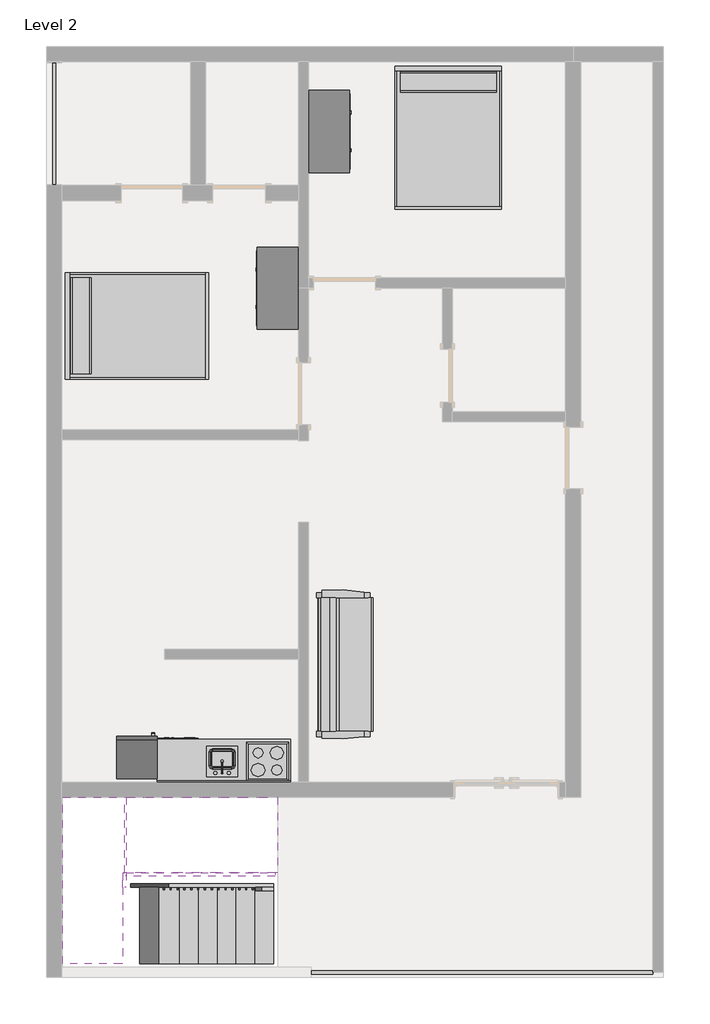
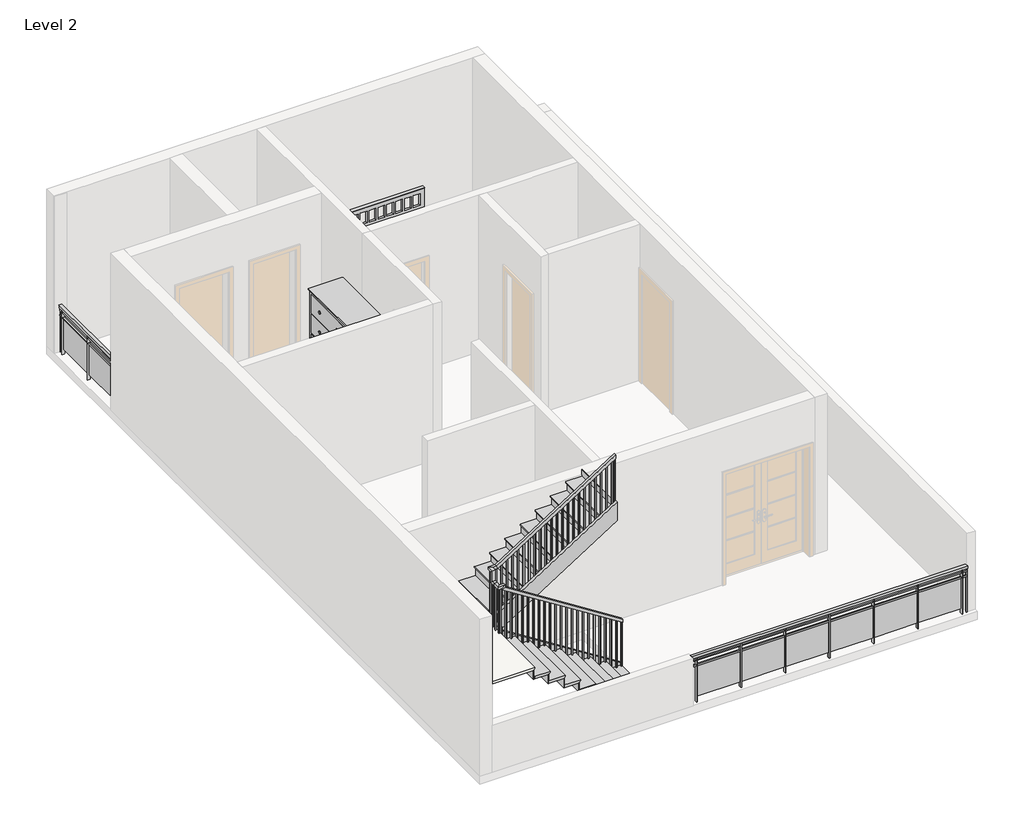
# One storey, part 2 of 2: 6 furniture elements, 4 proxies, 3 members, 3 railings, 2 stair flights, 1 flow terminal, 1 slab.
"""IFC4 building model written with IfcOpenShell, lengths in millimetres."""

from ifc_helpers import new_model, si_unit, frame, origin, place, context, project, spatial, polyline, outline, extrude, faceted_brep, transform, mapped, element, save
from components import proxy_a6faaae8, proxy_45b28599, kitchenette_medium_kitchenette_medium_844211aa, proxy_c523a7b7, flow_terminal_871c2e40, furniture_35c09872, furniture_c6510c7c, furniture_9fa109b2, furniture_aff9b2fb, non_monolithic_landing_077bd761, stair_flight_3c50d200, stair_flight_53bbb6a0

model = new_model("IFC4")

# Units and contexts
model_context = context("Model", 3, world=origin())
ifc_project = project(units=[si_unit("LENGTHUNIT", "METRE", prefix="MILLI")], contexts=[model_context])

# Site, building, storey
site = spatial("IfcSite", under=ifc_project)
building = spatial("IfcBuilding", under=site)
storey = spatial("IfcBuildingStorey", under=building, Name="Level 2", Elevation=3200.4)

# Proxies
placement = place(None, origin())
proxy_shape = proxy_a6faaae8(model_context)
element("IfcBuildingElementProxy", 1, Name="Cook Top-4 Unit2 : 22\" x 20\"", ObjectType="Cook Top-4 Unit2 : 22\" x 20\"", at=placement, inside=storey, context=model_context, shape_type="MappedRepresentation", body=[
    mapped(proxy_shape, transform((-8075.1683044, -841.1891189, 3200.4), x_axis=(-1.0000000000000004, 0.0, 0.0), y_axis=(0.0, -1.0000000000000004, 0.0), z_axis=(0.0, 0.0, 1.0))),
])
proxy_2_shape = proxy_45b28599(model_context)
element("IfcBuildingElementProxy", 2, Name="Dishwasher : 24\" x 24\" x 34\"", ObjectType="Dishwasher : 24\" x 24\" x 34\"", at=placement, inside=storey, context=model_context, shape_type="MappedRepresentation", body=[
    mapped(proxy_2_shape, transform((-9026.3508359, -549.3395541, 3200.4), x_axis=(-1.0000000000000004, 0.0, 0.0), y_axis=(0.0, -1.0000000000000004, 0.0), z_axis=(0.0, 0.0, 1.0))),
])
kitchenette_medium_kitchenette_medium_shape = kitchenette_medium_kitchenette_medium_844211aa(model_context)
element("IfcBuildingElementProxy", 3, Name="Kitchenette - Medium : Kitchenette - Medium", ObjectType="Kitchenette - Medium : Kitchenette - Medium", at=placement, inside=storey, context=model_context, shape_type="MappedRepresentation", body=[
    mapped(kitchenette_medium_kitchenette_medium_shape, transform((-8399.3305994, -1145.9891189, 3200.4), x_axis=(-1.0000000000000004, 0.0, 0.0), y_axis=(0.0, -1.0000000000000004, 0.0), z_axis=(0.0, 0.0, 1.0))),
])
proxy_3_shape = proxy_c523a7b7(model_context)
element("IfcBuildingElementProxy", 4, Name="Refrigerator : 24\" x 25\" LH", ObjectType="Refrigerator : 24\" x 25\" LH", at=placement, inside=storey, context=model_context, shape_type="MappedRepresentation", body=[
    mapped(proxy_3_shape, transform((-10011.9183044, -795.5401474, 3200.4), x_axis=(-1.0000000000000004, 0.0, 0.0), y_axis=(0.0, -1.0000000000000004, 0.0), z_axis=(0.0, 0.0, 1.0))),
])

# Flow terminal
flow_terminal_shape = flow_terminal_871c2e40(model_context)
element("IfcFlowTerminal", 5, ObjectType="Sink Kitchen-Island : 18\" x 18\"", at=placement, inside=storey, context=model_context, shape_type="MappedRepresentation", body=[
    mapped(flow_terminal_shape, transform((-8732.5790638, -838.8437178, 3186.0), x_axis=(-1.0000000000000004, 0.0, 0.0), y_axis=(0.0, -1.0000000000000004, 0.0), z_axis=(0.0, 0.0, 1.0))),
])

# Furniture
furniture_shape = furniture_35c09872(model_context)
element("IfcFurniture", 6, ObjectType="Bed-Shaker : Queen 62\" x 83\"", at=placement, inside=storey, context=model_context, shape_type="MappedRepresentation", body=[
    mapped(furniture_shape, transform((-11059.6683044, 5629.4608811, 3200.4), x_axis=(0.0, 1.0, 0.0), y_axis=(-1.0, 0.0, 0.0), z_axis=(0.0, 0.0, 1.0))),
])
element("IfcFurniture", 7, ObjectType="Bed-Shaker : Queen 62\" x 83\"", at=placement, inside=storey, context=model_context, shape_type="MappedRepresentation", body=[
    mapped(furniture_shape, transform((-5376.4183044, 9445.8108811, 3200.4), x_axis=(1.0, 0.0, 0.0), y_axis=(0.0, 1.0, 0.0), z_axis=(0.0, 0.0, 1.0))),
])
furniture_2_shape = furniture_c6510c7c(model_context)
element("IfcFurniture", 8, ObjectType="Counter Top w Sink Hole : 24\" Depth", at=placement, inside=storey, context=model_context, shape_type="MappedRepresentation", body=[
    mapped(furniture_2_shape, transform((-8932.7305994, -1145.9891189, 3186.0), x_axis=(-1.0000000000000004, 0.0, 0.0), y_axis=(0.0, -1.0000000000000004, 0.0), z_axis=(0.0, 0.0, 1.0))),
])
furniture_3_shape = furniture_9fa109b2(model_context)
element("IfcFurniture", 9, ObjectType="Dresser : 48\" x 72\" x 24\"", at=placement, inside=storey, context=model_context, shape_type="MappedRepresentation", body=[
    mapped(furniture_3_shape, transform((-7559.6053503, 5900.0176213, 3200.4), x_axis=(0.0, -1.0000000000000004, 0.0), y_axis=(1.0000000000000004, 0.0, 0.0), z_axis=(0.0, 0.0, 1.0))),
])
element("IfcFurniture", 10, ObjectType="Dresser : 48\" x 72\" x 24\"", at=placement, inside=storey, context=model_context, shape_type="MappedRepresentation", body=[
    mapped(furniture_3_shape, transform((-7523.9312585, 8762.5041409, 3200.4), x_axis=(0.0, 1.0000000000000009, 0.0), y_axis=(-1.0000000000000009, 0.0, 0.0), z_axis=(0.0, 0.0, 1.0))),
])
furniture_4_shape = furniture_aff9b2fb(model_context)
element("IfcFurniture", 11, ObjectType="Sofa-Pensi : 84\"", at=placement, inside=storey, context=model_context, shape_type="MappedRepresentation", body=[
    mapped(furniture_4_shape, transform((-6655.0584683, 315.3046311, 3200.4), x_axis=(0.0, 1.0, 0.0), y_axis=(-1.0, 0.0, 0.0), z_axis=(0.0, 0.0, 1.0))),
])

# Members
element("IfcMember", 12, ObjectType="Stringer - 2\" Width", at=placement, inside=storey, context=model_context, shape_type="SweptSolid", body=[
    extrude(outline(polyline([(3200.4, -7986.2683044), (3415.4106437, -7986.2683044), (4805.483371, -10170.6683044), (4444.2010268, -10170.6683044), (3200.4, -8216.1238337), (3200.4, -7986.2683044)])), frame((0.0, -2706.1923176, 0.0), z_axis=(0.0, 1.0, 0.0), x_axis=(0.0, 0.0, 1.0)), (0.0, 0.0, 1.0), 50.8),
])
element("IfcMember", 13, ObjectType="Stringer - 2\" Width", at=placement, inside=storey, context=model_context, shape_type="SweptSolid", body=[
    extrude(outline(polyline([(5031.7742801, -10170.6683044), (4670.4919359, -10170.6683044), (6076.7282995, -7960.8683044), (6438.0106437, -7960.8683044), (5031.7742801, -10170.6683044)])), frame((0.0, -2542.9891189, 0.0), z_axis=(0.0, 1.0, 0.0), x_axis=(0.0, 0.0, 1.0)), (0.0, 0.0, 1.0), 50.8),
])
element("IfcMember", 14, ObjectType="Stringer - 2\" Width", at=placement, inside=storey, context=model_context, shape_type="SweptSolid", body=[
    extrude(outline(polyline([(-10170.6683044, -2706.1923176), (-10221.4683044, -2706.1923176), (-10221.4683044, -2492.1891189), (-10170.6683044, -2492.1891189), (-10170.6683044, -2706.1923176)])), frame((0.0, 0.0, 4572.0), z_axis=(0.0, 0.0, 1.0), x_axis=(1.0, 0.0, 0.0)), (0.0, 0.0, 1.0), 304.8),
])

# Railings
element("IfcRailing", 15, ObjectType="Glass Panel - Bottom Fill", at=placement, inside=storey, context=model_context, shape_type="SweptSolid", body=[
    extrude(outline(polyline([(-7427.4683044, -3990.7891189), (-7427.4683044, -3939.9891189), (-2360.1683044, -3939.9891189), (-2360.1683044, -3990.7891189), (-7427.4683044, -3990.7891189)])), frame((0.0, 0.0, 4064.0), z_axis=(0.0, 0.0, 1.0), x_axis=(1.0, 0.0, 0.0)), (0.0, 0.0, 1.0), 50.8),
    extrude(outline(polyline([(-7427.4683044, -3978.0891189), (-7427.4683044, -3952.6891189), (-2360.1683044, -3952.6891189), (-2360.1683044, -3978.0891189), (-7427.4683044, -3978.0891189)])), frame((0.0, 0.0, 4000.5), z_axis=(0.0, 0.0, 1.0), x_axis=(1.0, 0.0, 0.0)), (0.0, 0.0, 1.0), 25.4),
    extrude(outline(polyline([(-7427.4683044, -3978.0891189), (-7427.4683044, -3952.6891189), (-2360.1683044, -3952.6891189), (-2360.1683044, -3978.0891189), (-7427.4683044, -3978.0891189)])), frame((0.0, 0.0, 3898.9), z_axis=(0.0, 0.0, 1.0), x_axis=(1.0, 0.0, 0.0)), (0.0, 0.0, 1.0), 25.4),
    extrude(outline(polyline([(-2461.7683044, -3990.7891189), (-2461.7683044, -3939.9891189), (-2449.0683044, -3939.9891189), (-2449.0683044, -3990.7891189), (-2461.7683044, -3990.7891189)])), frame((0.0, 0.0, 3200.4), z_axis=(0.0, 0.0, 1.0), x_axis=(1.0, 0.0, 0.0)), (0.0, 0.0, 1.0), 863.6),
    extrude(outline(polyline([(-3268.2183044, -3958.8539619), (-2455.4183044, -3958.8539619), (-2455.4183044, -3965.2039619), (-3268.2183044, -3965.2039619), (-3268.2183044, -3958.8539619)])), frame((0.0, 0.0, 3302.0), z_axis=(0.0, 0.0, 1.0), x_axis=(1.0, 0.0, 0.0)), (0.0, 0.0, 1.0), 596.9),
    extrude(outline(polyline([(-3274.5683044, -3990.7891189), (-3274.5683044, -3939.9891189), (-3261.8683044, -3939.9891189), (-3261.8683044, -3990.7891189), (-3274.5683044, -3990.7891189)])), frame((0.0, 0.0, 3200.4), z_axis=(0.0, 0.0, 1.0), x_axis=(1.0, 0.0, 0.0)), (0.0, 0.0, 1.0), 863.6),
    extrude(outline(polyline([(-4081.0183044, -3958.8539619), (-3268.2183044, -3958.8539619), (-3268.2183044, -3965.2039619), (-4081.0183044, -3965.2039619), (-4081.0183044, -3958.8539619)])), frame((0.0, 0.0, 3302.0), z_axis=(0.0, 0.0, 1.0), x_axis=(1.0, 0.0, 0.0)), (0.0, 0.0, 1.0), 596.9),
    extrude(outline(polyline([(-4087.3683044, -3990.7891189), (-4087.3683044, -3939.9891189), (-4074.6683044, -3939.9891189), (-4074.6683044, -3990.7891189), (-4087.3683044, -3990.7891189)])), frame((0.0, 0.0, 3200.4), z_axis=(0.0, 0.0, 1.0), x_axis=(1.0, 0.0, 0.0)), (0.0, 0.0, 1.0), 863.6),
    extrude(outline(polyline([(-4893.8183044, -3958.8539619), (-4081.0183044, -3958.8539619), (-4081.0183044, -3965.2039619), (-4893.8183044, -3965.2039619), (-4893.8183044, -3958.8539619)])), frame((0.0, 0.0, 3302.0), z_axis=(0.0, 0.0, 1.0), x_axis=(1.0, 0.0, 0.0)), (0.0, 0.0, 1.0), 596.9),
    extrude(outline(polyline([(-4900.1683044, -3990.7891189), (-4900.1683044, -3939.9891189), (-4887.4683044, -3939.9891189), (-4887.4683044, -3990.7891189), (-4900.1683044, -3990.7891189)])), frame((0.0, 0.0, 3200.4), z_axis=(0.0, 0.0, 1.0), x_axis=(1.0, 0.0, 0.0)), (0.0, 0.0, 1.0), 863.6),
    extrude(outline(polyline([(-5706.6183044, -3958.8539619), (-4893.8183044, -3958.8539619), (-4893.8183044, -3965.2039619), (-5706.6183044, -3965.2039619), (-5706.6183044, -3958.8539619)])), frame((0.0, 0.0, 3302.0), z_axis=(0.0, 0.0, 1.0), x_axis=(1.0, 0.0, 0.0)), (0.0, 0.0, 1.0), 596.9),
    extrude(outline(polyline([(-5712.9683044, -3990.7891189), (-5712.9683044, -3939.9891189), (-5700.2683044, -3939.9891189), (-5700.2683044, -3990.7891189), (-5712.9683044, -3990.7891189)])), frame((0.0, 0.0, 3200.4), z_axis=(0.0, 0.0, 1.0), x_axis=(1.0, 0.0, 0.0)), (0.0, 0.0, 1.0), 863.6),
    extrude(outline(polyline([(-6519.4183044, -3958.8539619), (-5706.6183044, -3958.8539619), (-5706.6183044, -3965.2039619), (-6519.4183044, -3965.2039619), (-6519.4183044, -3958.8539619)])), frame((0.0, 0.0, 3302.0), z_axis=(0.0, 0.0, 1.0), x_axis=(1.0, 0.0, 0.0)), (0.0, 0.0, 1.0), 596.9),
    extrude(outline(polyline([(-6525.7683044, -3990.7891189), (-6525.7683044, -3939.9891189), (-6513.0683044, -3939.9891189), (-6513.0683044, -3990.7891189), (-6525.7683044, -3990.7891189)])), frame((0.0, 0.0, 3200.4), z_axis=(0.0, 0.0, 1.0), x_axis=(1.0, 0.0, 0.0)), (0.0, 0.0, 1.0), 863.6),
    extrude(outline(polyline([(-7332.2183044, -3958.8539619), (-6519.4183044, -3958.8539619), (-6519.4183044, -3965.2039619), (-7332.2183044, -3965.2039619), (-7332.2183044, -3958.8539619)])), frame((0.0, 0.0, 3302.0), z_axis=(0.0, 0.0, 1.0), x_axis=(1.0, 0.0, 0.0)), (0.0, 0.0, 1.0), 596.9),
    extrude(outline(polyline([(-7338.5683044, -3990.7891189), (-7338.5683044, -3939.9891189), (-7325.8683044, -3939.9891189), (-7325.8683044, -3990.7891189), (-7338.5683044, -3990.7891189)])), frame((0.0, 0.0, 3200.4), z_axis=(0.0, 0.0, 1.0), x_axis=(1.0, 0.0, 0.0)), (0.0, 0.0, 1.0), 863.6),
    extrude(outline(polyline([(-2372.8683044, -3974.9141189), (-2372.8683044, -3955.8641189), (-2353.8183044, -3955.8641189), (-2353.8183044, -3974.9141189), (-2372.8683044, -3974.9141189)])), frame((0.0, 0.0, 3200.4), z_axis=(0.0, 0.0, 1.0), x_axis=(1.0, 0.0, 0.0)), (0.0, 0.0, 1.0), 863.6),
    extrude(outline(polyline([(-7433.8183044, -3974.9141189), (-7433.8183044, -3955.8641189), (-7414.7683044, -3955.8641189), (-7414.7683044, -3974.9141189), (-7433.8183044, -3974.9141189)])), frame((0.0, 0.0, 3200.4), z_axis=(0.0, 0.0, 1.0), x_axis=(1.0, 0.0, 0.0)), (0.0, 0.0, 1.0), 863.6),
])
element("IfcRailing", 16, ObjectType="Glass Panel - Bottom Fill", at=placement, inside=storey, context=model_context, shape_type="SweptSolid", body=[
    extrude(outline(polyline([(-11262.8683044, 9509.3108811), (-11212.0683044, 9509.3108811), (-11212.0683044, 7705.9108811), (-11262.8683044, 7705.9108811), (-11262.8683044, 9509.3108811)])), frame((0.0, 0.0, 4064.0), z_axis=(0.0, 0.0, 1.0), x_axis=(1.0, 0.0, 0.0)), (0.0, 0.0, 1.0), 50.8),
    extrude(outline(polyline([(-11250.1683044, 9509.3108811), (-11224.7683044, 9509.3108811), (-11224.7683044, 7705.9108811), (-11250.1683044, 7705.9108811), (-11250.1683044, 9509.3108811)])), frame((0.0, 0.0, 4000.5), z_axis=(0.0, 0.0, 1.0), x_axis=(1.0, 0.0, 0.0)), (0.0, 0.0, 1.0), 25.4),
    extrude(outline(polyline([(-11250.1683044, 9509.3108811), (-11224.7683044, 9509.3108811), (-11224.7683044, 7705.9108811), (-11250.1683044, 7705.9108811), (-11250.1683044, 9509.3108811)])), frame((0.0, 0.0, 3898.9), z_axis=(0.0, 0.0, 1.0), x_axis=(1.0, 0.0, 0.0)), (0.0, 0.0, 1.0), 25.4),
    extrude(outline(polyline([(-11262.8683044, 7801.1608811), (-11212.0683044, 7801.1608811), (-11212.0683044, 7788.4608811), (-11262.8683044, 7788.4608811), (-11262.8683044, 7801.1608811)])), frame((0.0, 0.0, 3200.4), z_axis=(0.0, 0.0, 1.0), x_axis=(1.0, 0.0, 0.0)), (0.0, 0.0, 1.0), 863.6),
    extrude(outline(polyline([(-11230.9331474, 8607.6108811), (-11230.9331474, 7794.8108811), (-11237.2831474, 7794.8108811), (-11237.2831474, 8607.6108811), (-11230.9331474, 8607.6108811)])), frame((0.0, 0.0, 3302.0), z_axis=(0.0, 0.0, 1.0), x_axis=(1.0, 0.0, 0.0)), (0.0, 0.0, 1.0), 596.9),
    extrude(outline(polyline([(-11262.8683044, 8613.9608811), (-11212.0683044, 8613.9608811), (-11212.0683044, 8601.2608811), (-11262.8683044, 8601.2608811), (-11262.8683044, 8613.9608811)])), frame((0.0, 0.0, 3200.4), z_axis=(0.0, 0.0, 1.0), x_axis=(1.0, 0.0, 0.0)), (0.0, 0.0, 1.0), 863.6),
    extrude(outline(polyline([(-11230.9331474, 9420.4108811), (-11230.9331474, 8607.6108811), (-11237.2831474, 8607.6108811), (-11237.2831474, 9420.4108811), (-11230.9331474, 9420.4108811)])), frame((0.0, 0.0, 3302.0), z_axis=(0.0, 0.0, 1.0), x_axis=(1.0, 0.0, 0.0)), (0.0, 0.0, 1.0), 596.9),
    extrude(outline(polyline([(-11262.8683044, 9426.7608811), (-11212.0683044, 9426.7608811), (-11212.0683044, 9414.0608811), (-11262.8683044, 9414.0608811), (-11262.8683044, 9426.7608811)])), frame((0.0, 0.0, 3200.4), z_axis=(0.0, 0.0, 1.0), x_axis=(1.0, 0.0, 0.0)), (0.0, 0.0, 1.0), 863.6),
    extrude(outline(polyline([(-11246.9933044, 7718.6108811), (-11227.9433044, 7718.6108811), (-11227.9433044, 7699.5608811), (-11246.9933044, 7699.5608811), (-11246.9933044, 7718.6108811)])), frame((0.0, 0.0, 3200.4), z_axis=(0.0, 0.0, 1.0), x_axis=(1.0, 0.0, 0.0)), (0.0, 0.0, 1.0), 863.6),
    extrude(outline(polyline([(-11246.9933044, 9515.6608811), (-11227.9433044, 9515.6608811), (-11227.9433044, 9496.6108811), (-11246.9933044, 9496.6108811), (-11246.9933044, 9515.6608811)])), frame((0.0, 0.0, 3200.4), z_axis=(0.0, 0.0, 1.0), x_axis=(1.0, 0.0, 0.0)), (0.0, 0.0, 1.0), 863.6),
])
element("IfcRailing", 17, ObjectType="Handrail - Rectangular", at=placement, inside=storey, context=model_context, shape_type="SolidModel", body=[
    faceted_brep([(-7986.2683044, -2756.9923176, 4292.6), (-7986.2683044, -2756.9923176, 4232.386276), (-7986.2683044, -2706.1923176, 4232.386276), (-7986.2683044, -2706.1923176, 4292.6), (-10145.2683044, -2756.9923176, 5666.5090909), (-10196.0683044, -2756.9923176, 5638.6226396), (-10196.0683044, -2706.1923176, 5638.6226396), (-10145.2683044, -2706.1923176, 5666.5090909), (-10145.2683044, -2756.9923176, 5715.0), (-10196.0683044, -2756.9923176, 5664.2), (-10196.0683044, -2706.1923176, 5664.2), (-10145.2683044, -2706.1923176, 5715.0), (-10272.2683044, -2756.9923176, 5715.0), (-10272.2683044, -2756.9923176, 5664.2), (-10221.4683044, -2706.1923176, 5664.2), (-10221.4683044, -2706.1923176, 5715.0), (-10272.2683044, -2629.9923176, 5715.0), (-10272.2683044, -2629.9923176, 5664.2), (-10221.4683044, -2629.9923176, 5664.2), (-10221.4683044, -2629.9923176, 5715.0), (-10272.2683044, -2568.3891189, 5715.0), (-10272.2683044, -2517.5891189, 5664.2), (-10221.4683044, -2517.5891189, 5664.2), (-10221.4683044, -2568.3891189, 5715.0), (-10272.2683044, -2568.3891189, 5925.1272727), (-10272.2683044, -2517.5891189, 5874.3272727), (-10221.4683044, -2517.5891189, 5874.3272727), (-10221.4683044, -2568.3891189, 5925.1272727), (-7960.8683044, -2441.3891189, 7315.2), (-7960.8683044, -2492.1891189, 7315.2), (-7960.8683044, -2492.1891189, 7254.986276), (-7960.8683044, -2441.3891189, 7254.986276), (-10130.4753095, -2441.3891189, 5874.3272727), (-10145.2683044, -2441.3891189, 5925.1272727), (-10130.4753095, -2492.1891189, 5874.3272727), (-10145.2683044, -2492.1891189, 5925.1272727), (-10272.2683044, -2441.3891189, 5925.1272727), (-10272.2683044, -2441.3891189, 5874.3272727), (-10221.4683044, -2492.1891189, 5874.3272727), (-10221.4683044, -2492.1891189, 5925.1272727)], [[[0, 1, 2, 3]], [[1, 0, 4, 5]], [[2, 1, 5, 6]], [[3, 2, 6, 7]], [[0, 3, 7, 4]], [[5, 4, 8, 9]], [[6, 5, 9, 10]], [[7, 6, 10, 11]], [[4, 7, 11, 8]], [[9, 8, 12, 13]], [[10, 9, 13, 14]], [[11, 10, 14, 15]], [[8, 11, 15, 12]], [[13, 12, 16, 17]], [[14, 13, 17, 18]], [[15, 14, 18, 19]], [[12, 15, 19, 16]], [[17, 16, 20, 21]], [[18, 17, 21, 22]], [[19, 18, 22, 23]], [[16, 19, 23, 20]], [[21, 20, 24, 25]], [[22, 21, 25, 26]], [[23, 22, 26, 27]], [[20, 23, 27, 24]], [[28, 29, 30, 31]], [[32, 33, 28, 31]], [[34, 32, 31, 30]], [[35, 34, 30, 29]], [[33, 35, 29, 28]], [[25, 24, 36, 37]], [[26, 25, 37, 38]], [[27, 26, 38, 39]], [[24, 27, 39, 36]], [[37, 36, 33, 32]], [[38, 37, 32, 34]], [[39, 38, 34, 35]], [[36, 39, 35, 33]]]),
    extrude(outline(polyline([(7228.7203669, -8002.1433044), (7216.5976396, -8021.1933044), (6223.0, -8021.1933044), (6223.0, -8002.1433044), (7228.7203669, -8002.1433044)])), frame((0.0, -2476.3141189, 0.0), z_axis=(0.0, 1.0, 0.0), x_axis=(0.0, 0.0, 1.0)), (0.0, 0.0, 1.0), 19.05),
    extrude(outline(polyline([(7164.0658214, -8103.7433044), (7151.9430941, -8122.7933044), (6223.0, -8122.7933044), (6223.0, -8103.7433044), (7164.0658214, -8103.7433044)])), frame((0.0, -2476.3141189, 0.0), z_axis=(0.0, 1.0, 0.0), x_axis=(0.0, 0.0, 1.0)), (0.0, 0.0, 1.0), 19.05),
    extrude(outline(polyline([(7099.411276, -8205.3433044), (7087.2885487, -8224.3933044), (6223.0, -8224.3933044), (6223.0, -8205.3433044), (7099.411276, -8205.3433044)])), frame((0.0, -2476.3141189, 0.0), z_axis=(0.0, 1.0, 0.0), x_axis=(0.0, 0.0, 1.0)), (0.0, 0.0, 1.0), 19.05),
    extrude(outline(polyline([(7034.7567305, -8306.9433044), (7022.6340032, -8325.9933044), (6045.2, -8325.9933044), (6045.2, -8306.9433044), (7034.7567305, -8306.9433044)])), frame((0.0, -2476.3141189, 0.0), z_axis=(0.0, 1.0, 0.0), x_axis=(0.0, 0.0, 1.0)), (0.0, 0.0, 1.0), 19.05),
    extrude(outline(polyline([(6970.1021851, -8408.5433044), (6957.9794578, -8427.5933044), (6045.2, -8427.5933044), (6045.2, -8408.5433044), (6970.1021851, -8408.5433044)])), frame((0.0, -2476.3141189, 0.0), z_axis=(0.0, 1.0, 0.0), x_axis=(0.0, 0.0, 1.0)), (0.0, 0.0, 1.0), 19.05),
    extrude(outline(polyline([(6905.4476396, -8510.1433044), (6893.3249123, -8529.1933044), (6045.2, -8529.1933044), (6045.2, -8510.1433044), (6905.4476396, -8510.1433044)])), frame((0.0, -2476.3141189, 0.0), z_axis=(0.0, 1.0, 0.0), x_axis=(0.0, 0.0, 1.0)), (0.0, 0.0, 1.0), 19.05),
    extrude(outline(polyline([(6840.7930941, -8611.7433044), (6828.6703669, -8630.7933044), (5867.4, -8630.7933044), (5867.4, -8611.7433044), (6840.7930941, -8611.7433044)])), frame((0.0, -2476.3141189, 0.0), z_axis=(0.0, 1.0, 0.0), x_axis=(0.0, 0.0, 1.0)), (0.0, 0.0, 1.0), 19.05),
    extrude(outline(polyline([(6776.1385487, -8713.3433044), (6764.0158214, -8732.3933044), (5867.4, -8732.3933044), (5867.4, -8713.3433044), (6776.1385487, -8713.3433044)])), frame((0.0, -2476.3141189, 0.0), z_axis=(0.0, 1.0, 0.0), x_axis=(0.0, 0.0, 1.0)), (0.0, 0.0, 1.0), 19.05),
    extrude(outline(polyline([(6711.4840032, -8814.9433044), (6699.361276, -8833.9933044), (5689.6, -8833.9933044), (5689.6, -8814.9433044), (6711.4840032, -8814.9433044)])), frame((0.0, -2476.3141189, 0.0), z_axis=(0.0, 1.0, 0.0), x_axis=(0.0, 0.0, 1.0)), (0.0, 0.0, 1.0), 19.05),
    extrude(outline(polyline([(6646.8294578, -8916.5433044), (6634.7067305, -8935.5933044), (5689.6, -8935.5933044), (5689.6, -8916.5433044), (6646.8294578, -8916.5433044)])), frame((0.0, -2476.3141189, 0.0), z_axis=(0.0, 1.0, 0.0), x_axis=(0.0, 0.0, 1.0)), (0.0, 0.0, 1.0), 19.05),
    extrude(outline(polyline([(6582.1749123, -9018.1433044), (6570.0521851, -9037.1933044), (5689.6, -9037.1933044), (5689.6, -9018.1433044), (6582.1749123, -9018.1433044)])), frame((0.0, -2476.3141189, 0.0), z_axis=(0.0, 1.0, 0.0), x_axis=(0.0, 0.0, 1.0)), (0.0, 0.0, 1.0), 19.05),
    extrude(outline(polyline([(6517.5203669, -9119.7433044), (6505.3976396, -9138.7933044), (5511.8, -9138.7933044), (5511.8, -9119.7433044), (6517.5203669, -9119.7433044)])), frame((0.0, -2476.3141189, 0.0), z_axis=(0.0, 1.0, 0.0), x_axis=(0.0, 0.0, 1.0)), (0.0, 0.0, 1.0), 19.05),
    extrude(outline(polyline([(6452.8658214, -9221.3433044), (6440.7430941, -9240.3933044), (5511.8, -9240.3933044), (5511.8, -9221.3433044), (6452.8658214, -9221.3433044)])), frame((0.0, -2476.3141189, 0.0), z_axis=(0.0, 1.0, 0.0), x_axis=(0.0, 0.0, 1.0)), (0.0, 0.0, 1.0), 19.05),
    extrude(outline(polyline([(6388.211276, -9322.9433044), (6376.0885487, -9341.9933044), (5511.8, -9341.9933044), (5511.8, -9322.9433044), (6388.211276, -9322.9433044)])), frame((0.0, -2476.3141189, 0.0), z_axis=(0.0, 1.0, 0.0), x_axis=(0.0, 0.0, 1.0)), (0.0, 0.0, 1.0), 19.05),
    extrude(outline(polyline([(6323.5567305, -9424.5433044), (6311.4340032, -9443.5933044), (5334.0, -9443.5933044), (5334.0, -9424.5433044), (6323.5567305, -9424.5433044)])), frame((0.0, -2476.3141189, 0.0), z_axis=(0.0, 1.0, 0.0), x_axis=(0.0, 0.0, 1.0)), (0.0, 0.0, 1.0), 19.05),
    extrude(outline(polyline([(6258.9021851, -9526.1433044), (6246.7794578, -9545.1933044), (5334.0, -9545.1933044), (5334.0, -9526.1433044), (6258.9021851, -9526.1433044)])), frame((0.0, -2476.3141189, 0.0), z_axis=(0.0, 1.0, 0.0), x_axis=(0.0, 0.0, 1.0)), (0.0, 0.0, 1.0), 19.05),
    extrude(outline(polyline([(6194.2476396, -9627.7433044), (6182.1249123, -9646.7933044), (5334.0, -9646.7933044), (5334.0, -9627.7433044), (6194.2476396, -9627.7433044)])), frame((0.0, -2476.3141189, 0.0), z_axis=(0.0, 1.0, 0.0), x_axis=(0.0, 0.0, 1.0)), (0.0, 0.0, 1.0), 19.05),
    extrude(outline(polyline([(6129.5930941, -9729.3433044), (6117.4703669, -9748.3933044), (5156.2, -9748.3933044), (5156.2, -9729.3433044), (6129.5930941, -9729.3433044)])), frame((0.0, -2476.3141189, 0.0), z_axis=(0.0, 1.0, 0.0), x_axis=(0.0, 0.0, 1.0)), (0.0, 0.0, 1.0), 19.05),
    extrude(outline(polyline([(6064.9385487, -9830.9433044), (6052.8158214, -9849.9933044), (5156.2, -9849.9933044), (5156.2, -9830.9433044), (6064.9385487, -9830.9433044)])), frame((0.0, -2476.3141189, 0.0), z_axis=(0.0, 1.0, 0.0), x_axis=(0.0, 0.0, 1.0)), (0.0, 0.0, 1.0), 19.05),
    extrude(outline(polyline([(6000.2840032, -9932.5433044), (5988.161276, -9951.5933044), (4978.4, -9951.5933044), (4978.4, -9932.5433044), (6000.2840032, -9932.5433044)])), frame((0.0, -2476.3141189, 0.0), z_axis=(0.0, 1.0, 0.0), x_axis=(0.0, 0.0, 1.0)), (0.0, 0.0, 1.0), 19.05),
    extrude(outline(polyline([(5935.6294578, -10034.1433044), (5923.5067305, -10053.1933044), (4978.4, -10053.1933044), (4978.4, -10034.1433044), (5935.6294578, -10034.1433044)])), frame((0.0, -2476.3141189, 0.0), z_axis=(0.0, 1.0, 0.0), x_axis=(0.0, 0.0, 1.0)), (0.0, 0.0, 1.0), 19.05),
    extrude(outline(polyline([(-10154.7933044, -2476.3141189), (-10154.7933044, -2457.2641189), (-10135.7433044, -2457.2641189), (-10135.7433044, -2476.3141189), (-10154.7933044, -2476.3141189)])), frame((0.0, 0.0, 4978.4), z_axis=(0.0, 0.0, 1.0), x_axis=(1.0, 0.0, 0.0)), (0.0, 0.0, 1.0), 895.9272727),
    extrude(outline(polyline([(-10237.3433044, -2537.9173176), (-10256.3933044, -2537.9173176), (-10256.3933044, -2518.8673176), (-10237.3433044, -2518.8673176), (-10237.3433044, -2537.9173176)])), frame((0.0, 0.0, 4800.6), z_axis=(0.0, 0.0, 1.0), x_axis=(1.0, 0.0, 0.0)), (0.0, 0.0, 1.0), 863.6),
    extrude(outline(polyline([(-10237.3433044, -2639.5173176), (-10256.3933044, -2639.5173176), (-10256.3933044, -2620.4673176), (-10237.3433044, -2620.4673176), (-10237.3433044, -2639.5173176)])), frame((0.0, 0.0, 4800.6), z_axis=(0.0, 0.0, 1.0), x_axis=(1.0, 0.0, 0.0)), (0.0, 0.0, 1.0), 863.6),
    extrude(outline(polyline([(5584.0703669, -10110.3433044), (5596.1930941, -10129.3933044), (4622.8, -10129.3933044), (4622.8, -10110.3433044), (5584.0703669, -10110.3433044)])), frame((0.0, -2741.1173176, 0.0), z_axis=(0.0, 1.0, 0.0), x_axis=(0.0, 0.0, 1.0)), (0.0, 0.0, 1.0), 19.05),
    extrude(outline(polyline([(5519.4158214, -10008.7433044), (5531.5385487, -10027.7933044), (4622.8, -10027.7933044), (4622.8, -10008.7433044), (5519.4158214, -10008.7433044)])), frame((0.0, -2741.1173176, 0.0), z_axis=(0.0, 1.0, 0.0), x_axis=(0.0, 0.0, 1.0)), (0.0, 0.0, 1.0), 19.05),
    extrude(outline(polyline([(5454.761276, -9907.1433044), (5466.8840032, -9926.1933044), (4445.0, -9926.1933044), (4445.0, -9907.1433044), (5454.761276, -9907.1433044)])), frame((0.0, -2741.1173176, 0.0), z_axis=(0.0, 1.0, 0.0), x_axis=(0.0, 0.0, 1.0)), (0.0, 0.0, 1.0), 19.05),
    extrude(outline(polyline([(5390.1067305, -9805.5433044), (5402.2294578, -9824.5933044), (4445.0, -9824.5933044), (4445.0, -9805.5433044), (5390.1067305, -9805.5433044)])), frame((0.0, -2741.1173176, 0.0), z_axis=(0.0, 1.0, 0.0), x_axis=(0.0, 0.0, 1.0)), (0.0, 0.0, 1.0), 19.05),
    extrude(outline(polyline([(5325.4521851, -9703.9433044), (5337.5749123, -9722.9933044), (4445.0, -9722.9933044), (4445.0, -9703.9433044), (5325.4521851, -9703.9433044)])), frame((0.0, -2741.1173176, 0.0), z_axis=(0.0, 1.0, 0.0), x_axis=(0.0, 0.0, 1.0)), (0.0, 0.0, 1.0), 19.05),
    extrude(outline(polyline([(5260.7976396, -9602.3433044), (5272.9203669, -9621.3933044), (4267.2, -9621.3933044), (4267.2, -9602.3433044), (5260.7976396, -9602.3433044)])), frame((0.0, -2741.1173176, 0.0), z_axis=(0.0, 1.0, 0.0), x_axis=(0.0, 0.0, 1.0)), (0.0, 0.0, 1.0), 19.05),
    extrude(outline(polyline([(5196.1430941, -9500.7433044), (5208.2658214, -9519.7933044), (4267.2, -9519.7933044), (4267.2, -9500.7433044), (5196.1430941, -9500.7433044)])), frame((0.0, -2741.1173176, 0.0), z_axis=(0.0, 1.0, 0.0), x_axis=(0.0, 0.0, 1.0)), (0.0, 0.0, 1.0), 19.05),
    extrude(outline(polyline([(5131.4885487, -9399.1433044), (5143.611276, -9418.1933044), (4267.2, -9418.1933044), (4267.2, -9399.1433044), (5131.4885487, -9399.1433044)])), frame((0.0, -2741.1173176, 0.0), z_axis=(0.0, 1.0, 0.0), x_axis=(0.0, 0.0, 1.0)), (0.0, 0.0, 1.0), 19.05),
    extrude(outline(polyline([(5066.8340032, -9297.5433044), (5078.9567305, -9316.5933044), (4089.4, -9316.5933044), (4089.4, -9297.5433044), (5066.8340032, -9297.5433044)])), frame((0.0, -2741.1173176, 0.0), z_axis=(0.0, 1.0, 0.0), x_axis=(0.0, 0.0, 1.0)), (0.0, 0.0, 1.0), 19.05),
    extrude(outline(polyline([(5002.1794578, -9195.9433044), (5014.3021851, -9214.9933044), (4089.4, -9214.9933044), (4089.4, -9195.9433044), (5002.1794578, -9195.9433044)])), frame((0.0, -2741.1173176, 0.0), z_axis=(0.0, 1.0, 0.0), x_axis=(0.0, 0.0, 1.0)), (0.0, 0.0, 1.0), 19.05),
    extrude(outline(polyline([(4937.5249123, -9094.3433044), (4949.6476396, -9113.3933044), (4089.4, -9113.3933044), (4089.4, -9094.3433044), (4937.5249123, -9094.3433044)])), frame((0.0, -2741.1173176, 0.0), z_axis=(0.0, 1.0, 0.0), x_axis=(0.0, 0.0, 1.0)), (0.0, 0.0, 1.0), 19.05),
    extrude(outline(polyline([(4872.8703669, -8992.7433044), (4884.9930941, -9011.7933044), (3911.6, -9011.7933044), (3911.6, -8992.7433044), (4872.8703669, -8992.7433044)])), frame((0.0, -2741.1173176, 0.0), z_axis=(0.0, 1.0, 0.0), x_axis=(0.0, 0.0, 1.0)), (0.0, 0.0, 1.0), 19.05),
    extrude(outline(polyline([(4808.2158214, -8891.1433044), (4820.3385487, -8910.1933044), (3911.6, -8910.1933044), (3911.6, -8891.1433044), (4808.2158214, -8891.1433044)])), frame((0.0, -2741.1173176, 0.0), z_axis=(0.0, 1.0, 0.0), x_axis=(0.0, 0.0, 1.0)), (0.0, 0.0, 1.0), 19.05),
    extrude(outline(polyline([(4743.561276, -8789.5433044), (4755.6840032, -8808.5933044), (3733.8, -8808.5933044), (3733.8, -8789.5433044), (4743.561276, -8789.5433044)])), frame((0.0, -2741.1173176, 0.0), z_axis=(0.0, 1.0, 0.0), x_axis=(0.0, 0.0, 1.0)), (0.0, 0.0, 1.0), 19.05),
    extrude(outline(polyline([(4678.9067305, -8687.9433044), (4691.0294578, -8706.9933044), (3733.8, -8706.9933044), (3733.8, -8687.9433044), (4678.9067305, -8687.9433044)])), frame((0.0, -2741.1173176, 0.0), z_axis=(0.0, 1.0, 0.0), x_axis=(0.0, 0.0, 1.0)), (0.0, 0.0, 1.0), 19.05),
    extrude(outline(polyline([(4614.2521851, -8586.3433044), (4626.3749123, -8605.3933044), (3733.8, -8605.3933044), (3733.8, -8586.3433044), (4614.2521851, -8586.3433044)])), frame((0.0, -2741.1173176, 0.0), z_axis=(0.0, 1.0, 0.0), x_axis=(0.0, 0.0, 1.0)), (0.0, 0.0, 1.0), 19.05),
    extrude(outline(polyline([(4549.5976396, -8484.7433044), (4561.7203669, -8503.7933044), (3556.0, -8503.7933044), (3556.0, -8484.7433044), (4549.5976396, -8484.7433044)])), frame((0.0, -2741.1173176, 0.0), z_axis=(0.0, 1.0, 0.0), x_axis=(0.0, 0.0, 1.0)), (0.0, 0.0, 1.0), 19.05),
    extrude(outline(polyline([(4484.9430941, -8383.1433044), (4497.0658214, -8402.1933044), (3556.0, -8402.1933044), (3556.0, -8383.1433044), (4484.9430941, -8383.1433044)])), frame((0.0, -2741.1173176, 0.0), z_axis=(0.0, 1.0, 0.0), x_axis=(0.0, 0.0, 1.0)), (0.0, 0.0, 1.0), 19.05),
    extrude(outline(polyline([(4420.2885487, -8281.5433044), (4432.411276, -8300.5933044), (3556.0, -8300.5933044), (3556.0, -8281.5433044), (4420.2885487, -8281.5433044)])), frame((0.0, -2741.1173176, 0.0), z_axis=(0.0, 1.0, 0.0), x_axis=(0.0, 0.0, 1.0)), (0.0, 0.0, 1.0), 19.05),
    extrude(outline(polyline([(4355.6340032, -8179.9433044), (4367.7567305, -8198.9933044), (3378.2, -8198.9933044), (3378.2, -8179.9433044), (4355.6340032, -8179.9433044)])), frame((0.0, -2741.1173176, 0.0), z_axis=(0.0, 1.0, 0.0), x_axis=(0.0, 0.0, 1.0)), (0.0, 0.0, 1.0), 19.05),
    extrude(outline(polyline([(4290.9794578, -8078.3433044), (4303.1021851, -8097.3933044), (3378.2, -8097.3933044), (3378.2, -8078.3433044), (4290.9794578, -8078.3433044)])), frame((0.0, -2741.1173176, 0.0), z_axis=(0.0, 1.0, 0.0), x_axis=(0.0, 0.0, 1.0)), (0.0, 0.0, 1.0), 19.05),
    extrude(outline(polyline([(-10256.3933044, -2476.3141189), (-10256.3933044, -2457.2641189), (-10237.3433044, -2457.2641189), (-10237.3433044, -2476.3141189), (-10256.3933044, -2476.3141189)])), frame((0.0, 0.0, 4800.6), z_axis=(0.0, 0.0, 1.0), x_axis=(1.0, 0.0, 0.0)), (0.0, 0.0, 1.0), 1073.7272727),
    extrude(outline(polyline([(-10237.3433044, -2722.0673176), (-10237.3433044, -2741.1173176), (-10256.3933044, -2741.1173176), (-10256.3933044, -2722.0673176), (-10237.3433044, -2722.0673176)])), frame((0.0, 0.0, 4800.6), z_axis=(0.0, 0.0, 1.0), x_axis=(1.0, 0.0, 0.0)), (0.0, 0.0, 1.0), 863.6),
    extrude(outline(polyline([(-10211.9433044, -2722.0673176), (-10211.9433044, -2741.1173176), (-10230.9933044, -2741.1173176), (-10230.9933044, -2722.0673176), (-10211.9433044, -2722.0673176)])), frame((0.0, 0.0, 4800.6), z_axis=(0.0, 0.0, 1.0), x_axis=(1.0, 0.0, 0.0)), (0.0, 0.0, 1.0), 863.6),
    extrude(outline(polyline([(7254.986276, -7960.8683044), (7242.8635487, -7979.9183044), (6223.0, -7979.9183044), (6223.0, -7960.8683044), (7254.986276, -7960.8683044)])), frame((0.0, -2476.3141189, 0.0), z_axis=(0.0, 1.0, 0.0), x_axis=(0.0, 0.0, 1.0)), (0.0, 0.0, 1.0), 19.05),
    extrude(outline(polyline([(4232.386276, -7986.2683044), (4244.5090032, -8005.3183044), (3378.2, -8005.3183044), (3378.2, -7986.2683044), (4232.386276, -7986.2683044)])), frame((0.0, -2741.1173176, 0.0), z_axis=(0.0, 1.0, 0.0), x_axis=(0.0, 0.0, 1.0)), (0.0, 0.0, 1.0), 19.05),
])

# Slab
non_monolithic_landing_shape = non_monolithic_landing_077bd761(model_context)
element("IfcSlab", 18, ObjectType="Non-Monolithic Landing", at=placement, inside=storey, context=model_context, shape_type="MappedRepresentation", body=[
    mapped(non_monolithic_landing_shape, transform((0.0, 0.0, 0.0), x_axis=(1.0, 0.0, 0.0), y_axis=(0.0, 1.0, 0.0), z_axis=(0.0, 0.0, 1.0))),
])

# Stair flights
stair_flight_shape = stair_flight_3c50d200(model_context)
element("IfcStairFlight", 19, ObjectType="2\" Tread 1\" Nosing 1/4\" Riser", at=placement, inside=storey, context=model_context, shape_type="MappedRepresentation", body=[
    mapped(stair_flight_shape, transform((0.0, 0.0, 0.0), x_axis=(1.0, 0.0, 0.0), y_axis=(0.0, 1.0, 0.0), z_axis=(0.0, 0.0, 1.0))),
])
stair_flight_2_shape = stair_flight_53bbb6a0(model_context)
element("IfcStairFlight", 20, ObjectType="2\" Tread 1\" Nosing 1/4\" Riser", at=placement, inside=storey, context=model_context, shape_type="MappedRepresentation", body=[
    mapped(stair_flight_2_shape, transform((0.0, 0.0, 0.0), x_axis=(1.0, 0.0, 0.0), y_axis=(0.0, 1.0, 0.0), z_axis=(0.0, 0.0, 1.0))),
])

save(model, "model.ifc")

# Revit data of these elements
# Type "Cook Top-4 Unit2 : 22\" x 20\""
#   Depth = 1' - 8"
#   Width = 1' - 10"
#   Burner Material = Steel, Chrome Plated
#   Cooktop Material = Steel, Polished
#   Default Elevation = 0
#   Assembly Code = ""
# Type "Dishwasher : 24\" x 24\" x 34\""
#   Label = "DW"
#   Assembly Code = "E1090400"
#   Depth = 2' - 0"
#   Height = 2' - 10"
#   Width = 2' - 0"
#   Dishwasher Material = Steel, Paint Finish, Ivory, Glossy
#   Panel Face Material = Plastic, Opaque Black
#   Default Elevation = 0
# Type "Kitchenette - Medium : Kitchenette - Medium"
#   Assembly Code = "E1090400"
#   Counter Length = 6' - 6"
#   Cabinet Width = 4' - 6"
#   Cabinet Height = 2' - 10 1/2"
#   Cabinet Depth = 2' - 0"
#   Toe Depth = 0' - 3"
#   Toe Height = 0' - 3 1/2"
#   Cabinet Material = Cabinets
#   Door/Drawer Material = Cabinets
#   Handle Material = Cabinets - Handles
#   Default Elevation = 0
# Type "Refrigerator : 24\" x 25\" LH"
#   Label = "REF."
#   Assembly Code = "E1090400"
#   Depth = 2' - 0 3/4"
#   Handle = 0' - 1 1/2"
#   Height = 5' - 3 1/2"
#   Rear Clearance = 0' - 2"
#   Top Door Height = 1' - 8"
#   Width = 1' - 11 1/2"
#   Material = Steel, Paint Finish, Ivory, Glossy
#   Default Elevation = 0
# Type "Sink Kitchen-Island : 18\" x 18\""
#   Assembly Code = "D2010410"
#   Counter Height = 3' - 0"
#   Depth = 1' - 6"
#   Width = 1' - 6"
#   Faucet Material = Steel, Polished
#   Sink Material = Steel, Polished
#   Default Elevation = 0
# Type "Bed-Shaker : Queen 62\" x 83\""
#   Assembly Code = "E2020200"
#   Length = 6' - 11"
#   Width = 5' - 2"
#   Frame Material = Birch
#   Mattress Material = Linen, White
#   Default Elevation = 0
# Type "Counter Top w Sink Hole : 24\" Depth"
#   Assembly Code = "C1030400"
#   Counter Thickness = 0' - 1 1/2"
#   Depth = 2' - 1"
#   Height = 3' - 0"
#   Length [instance default] = 8' - 0"
#   Sink Location [instance default] = 2' - 0"
#   Sink Location To Wall [instance default] = 0' - 6"
#   Sink Opening Depth [instance default] = 1' - 3"
#   Sink Opening Width [instance default] = 2' - 3"
#   Counter Top Material = none
#   Default Elevation = 0
# Type "Dresser : 48\" x 72\" x 24\""
#   Assembly Code = "E2020200"
#   Depth = 2' - 0"
#   Height = 6' - 0"
#   Width = 4' - 0"
#   Dresser Material = Laminate - Ivory, Glossy
#   Drawer Material = Laminate, Ivory, Matte
#   Knob Material = Cherry
#   Default Elevation = 0
# Type "Sofa-Pensi : 84\""
#   Assembly Code = "E2020200"
#   Length = 7' - 0"
#   Frame Material = Cherry
#   Seat Material = Linen, Beige
#   Feet Material = Steel, Chrome Plated
#   Default Elevation = 0
# Type "Glass Panel - Bottom Fill"
#   Assembly Code = "C2010400"
#   built-in parameter 1008612 = 0.0416667 (stored number, unit not read)
#   built-in parameter 1008611 = 0.0416667 (stored number, unit not read)
#   built-in parameter 1008609 = 0.333333 (stored number, unit not read)
#   built-in parameter 1008604 = 0.166667 (stored number, unit not read)
#   built-in parameter 1008603 = 0.166667 (stored number, unit not read)
#   Railing Height = 3' - 0"
#   built-in parameter 1008630 = 2
#   built-in parameter 1008610 = 2
#   built-in parameter 1008618 = Baluster - Square : 3/4"
# Type "Handrail - Rectangular"
#   Assembly Code = "C2010400"
#   built-in parameter 1008612 = 0.0416667 (stored number, unit not read)
#   built-in parameter 1008611 = 0.0416667 (stored number, unit not read)
#   built-in parameter 1008609 = 0.333333 (stored number, unit not read)
#   built-in parameter 1008604 = 0.166667 (stored number, unit not read)
#   built-in parameter 1008603 = 0.166667 (stored number, unit not read)
#   Railing Height = 3' - 0"
#   built-in parameter 1008630 = 2
#   built-in parameter 1008610 = 2
#   built-in parameter 1008618 = Baluster - Square : 3/4"
# Element 1 (IfcBuildingElementProxy, "Cook Top-4 Unit2 : 22\" x 20\"")
#   Phase Created = New Construction
#   Materials on its faces: "Steel, Chrome Plated", "Steel, Polished"
# Element 2 (IfcBuildingElementProxy, "Dishwasher : 24\" x 24\" x 34\"")
#   Phase Created = New Construction
#   Materials on its faces: "Steel, Paint Finish, Ivory, Glossy", "Plastic, Opaque Black"
# Element 3 (IfcBuildingElementProxy, "Kitchenette - Medium : Kitchenette - Medium")
#   Phase Created = New Construction
#   Materials on its faces: "Cabinets", "Cabinets - Handles"
# Element 4 (IfcBuildingElementProxy, "Refrigerator : 24\" x 25\" LH")
#   Phase Created = New Construction
#   Materials on its faces: "Steel, Paint Finish, Ivory, Glossy", "Steel, Chrome Plated"
# Element 5 (IfcFlowTerminal, "Sink Kitchen-Island : 18\" x 18\"")
#   Mark = "6"
#   Phase Created = New Construction
#   Materials on its faces: "Steel, Polished"
# Elements 6, 7 (IfcFurniture, "Bed-Shaker : Queen 62\" x 83\"")
#   Phase Created = New Construction
#   Materials on its faces: "Birch", "Linen, White"
# Element 8 (IfcFurniture, "Counter Top w Sink Hole : 24\" Depth")
#   Sink Opening Depth = 1' - 2"
#   Sink Location To Wall = 0' - 6"
#   Length = 6' - 6"
#   Sink Location = 3' - 4"
#   Sink Opening Width = 1' - 4"
#   Phase Created = New Construction
#   Materials on its faces: "Counter Top"
# Elements 9, 10 (IfcFurniture, "Dresser : 48\" x 72\" x 24\"")
#   Phase Created = New Construction
#   Materials on its faces: "Laminate, Ivory, Matte", "Cherry", "Laminate - Ivory, Glossy"
# Element 11 (IfcFurniture, "Sofa-Pensi : 84\"")
#   Phase Created = New Construction
#   Materials on its faces: "Cherry", "Linen, Beige", "Steel, Chrome Plated"
# Elements 12, 13, 14 (IfcMember, "Stringer - 2\" Width")
#   Phase Created = New Construction
# Elements 15, 16 (IfcRailing, "Glass Panel - Bottom Fill")
#   Phase Created = New Construction
#   Materials on its faces: "Glass"
# Element 17 (IfcRailing, "Handrail - Rectangular")
#   Phase Created = New Construction
# Element 18 (IfcSlab, "Non-Monolithic Landing")
#   Phase Created = New Construction
# Elements 19, 20 (IfcStairFlight, "2\" Tread 1\" Nosing 1/4\" Riser")
#   Phase Created = New Construction
# Materials
#   "Steel, Chrome Plated": class "Metal", colour RGB 17 17 17, transparency 0, Description = "Chromiuim plated steel", Cost = 0
#   "Steel, Polished": class "Metal", colour RGB 57 57 57, transparency 0, Description = "Polished steel", Cost = 0
#   "Steel, Paint Finish, Ivory, Glossy": class "Metal", colour RGB 247 247 239, transparency 0, Description = "Steel, paint finish, ivory, glossy", Cost = 0
#   "Plastic, Opaque Black": class "Plastic", colour RGB 0 0 0, transparency 0.7, Description = "Plastic, generic, opaque black", Cost = 0
#   "Cabinets": colour RGB 249 249 249, transparency 0
#   "Cabinets - Handles": class "Metal", colour RGB 57 57 57, transparency 0
#   "Birch": class "Wood", colour RGB 224 178 126, transparency 0, Description = "Betula Alleghaniensis", Cost = 0
#   "Linen, White": class "Textile", colour RGB 247 247 239, transparency 0, Description = "Linen, white", Cost = 0
#   "Laminate - Ivory, Glossy": colour RGB 247 247 239, transparency 0
#   "Laminate, Ivory, Matte": class "Plastic", colour RGB 247 247 239, transparency 0, Description = "Plastic Laminate - Ivory, Matte", Cost = 0
#   "Cherry": class "Wood", colour RGB 226 177 128, transparency 0, Description = "Prunus Serotina", Cost = 0
#   "Linen, Beige": class "Textile", colour RGB 249 239 230, transparency 0, Description = "Linen, beige", Cost = 0
#   "Counter Top": class "Wood", colour RGB 226 177 128, transparency 0
#   "Glass": class "Glass", colour RGB 0 128 192, transparency 0.75, Description = "Soda Lime Glass", Cost = 0
